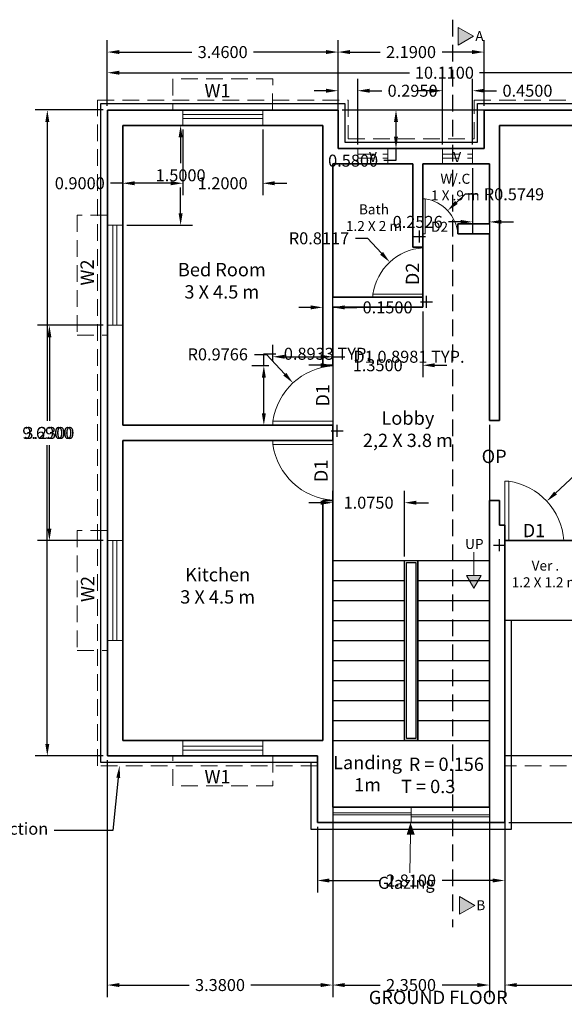
# Model space of a CAD drawing. Units: metres. Extents: x 5.2 to 41.7, y 12.2 to 37.4.
# Tile 3 of 6: x 19.4 to 27.6, y 12.2 to 27. Entities that reach past the tile are written whole.
import ezdxf
from ezdxf import colors
from ezdxf.entities.mleader import LeaderData, LeaderLine
from ezdxf.math import Vec2, Vec3

# ---------------------------------------------------------------- set-up
doc = ezdxf.new("R2010")
doc.units = ezdxf.units.M
doc.header["$MEASUREMENT"] = 0
doc.linetypes.add('HIDDEN', pattern=[0.375, 0.25, -0.125])
for name, color, linetype, lineweight in [('A-ANNO-DIMS', 2, 'Continuous', 18), ('A-ANNO-SYMB', 1, 'Continuous', 18), ('A-ANNO-SYMB-CUT', 3, 'HIDDEN', 25), ('A-ANNO-TEXT', 3, 'Continuous', 18), ('A-AREA-IDEN', 3, 'Continuous', 18), ('A-DOOR', 4, 'Continuous', 18), ('A-FLOR-PLIN', 7, 'Continuous', 25), ('A-FLOR-STRS', 7, 'Continuous', 25), ('A-ROOF-OVHD', 252, 'HIDDEN', 18), ('A-WALL', 7, 'Continuous', 35)]:
    doc.layers.add(name, color=color, linetype=linetype, lineweight=lineweight)
doc.layers.add('A-GLAZ', color=51, linetype='Continuous', lineweight=18, true_color=0xf7f281)
doc.layers.add('A-GLAZ-HIDN', color=51, linetype='HIDDEN', lineweight=18, true_color=0xf7f281)
doc.styles.get("Standard").update_dxf_attribs({"font": 'arial.ttf'})
doc.dimstyles.get("Standard").update_dxf_attribs({"dimtxt": 0.18, "dimasz": 0.18, "dimexe": 0.18, "dimexo": 0.0625, "dimgap": 0.09, "dimtad": 0, "dimtih": 1, "dimtoh": 1, "dimdec": 4, "dimzin": 0, "dimdsep": 46, "dimtxsty": 'Standard', "dimcen": 0.09, "dimadec": 0, "dimazin": 0, "dimtfac": 1, "dimtdec": 4, "dimtofl": 0, "dimtmove": 0, "dimatfit": 3, "dimfxl": 1, "dimtolj": 1, "dimtzin": 0, "dimarcsym": 0})

# ---------------------------------------------------------------- blocks, each defined once
blk = doc.blocks.new('*D2')
at = {"layer": 'A-ANNO-DIMS', "color": 0, "lineweight": -2, "transparency": 16777216}
for p, q in [((20.691, 25.661), (19.673, 25.661)), ((19.853, 25.481), (19.853, 20.998)), ((19.853, 16.151), (19.853, 20.634)), ((20.691, 15.971), (19.673, 15.971))]:
    blk.add_line(p, q, dxfattribs=at)
at = {"layer": 'A-ANNO-DIMS', "color": 0, "lineweight": 25, "transparency": 16777216}
for points in [[(19.823, 25.481), (19.883, 25.481), (19.853, 25.661)], [(19.823, 16.151), (19.883, 16.151), (19.853, 15.971)]]:
    blk.add_solid(points, dxfattribs=at)
at = {"layer": 'Defpoints', "color": 0, "lineweight": 25, "transparency": 16777216}
for p in [(19.853, 25.661), (20.753, 25.661), (20.753, 15.971)]:
    blk.add_point(p, dxfattribs=at)
at = {"layer": 'A-ANNO-DIMS', "color": 0, "transparency": 16777216, "insert": (19.853, 20.816), "char_height": 0.18, "attachment_point": 5}
blk.add_mtext('\\A1;9.6900', dxfattribs=at)
blk = doc.blocks.new('*D3')
at = {"layer": 'A-ANNO-DIMS', "color": 0, "lineweight": -2, "transparency": 16777216}
for p, q in [((20.753, 25.723), (20.753, 26.4)), ((30.863, 25.723), (30.863, 26.4)), ((20.933, 26.22), (25.283, 26.22)), ((30.683, 26.22), (26.333, 26.22))]:
    blk.add_line(p, q, dxfattribs=at)
at = {"layer": 'A-ANNO-DIMS', "color": 0, "lineweight": 25, "transparency": 16777216}
for points in [[(20.933, 26.25), (20.933, 26.19), (20.753, 26.22)], [(30.683, 26.25), (30.683, 26.19), (30.863, 26.22)]]:
    blk.add_solid(points, dxfattribs=at)
at = {"layer": 'Defpoints', "color": 0, "lineweight": 25, "transparency": 16777216}
for p in [(30.863, 26.22), (20.753, 25.661), (30.863, 25.661)]:
    blk.add_point(p, dxfattribs=at)
at = {"layer": 'A-ANNO-DIMS', "color": 0, "transparency": 16777216, "insert": (25.808, 26.22), "char_height": 0.18, "attachment_point": 5}
blk.add_mtext('\\A1;10.1100', dxfattribs=at)
blk = doc.blocks.new('WIN-W2-1500')
for p, q in [((0.23, 1.5), (0, 1.5)), ((0.085, 1.5), (0.085, 0)), ((0.145, 1.5), (0.145, 0)), ((0.23, 0), (0, 0))]:
    blk.add_line(p, q)
blk = doc.blocks.new('SUNSHADE-W2-1800')
blk.add_lwpolyline([(0.45, 1.65), (0.45, 1.8), (0, 1.8), (0, 0), (0.45, 0), (0.45, 0.15)])
blk = doc.blocks.new('DOOR-D1-900')
blk.add_lwpolyline([(0, 0), (0, 0.06), (0.898, 0.06), (0.898, 0)], close=True)
blk.add_arc((0.967, -0.081), 0.977, 94.015, 171.7193)
blk = doc.blocks.new('SECTION-DIRECTION')
h = blk.add_hatch(color=256)
h.dxf.hatch_style = 1
h.paths.add_polyline_path([(0, 0.266), (0, 0), (0.231, 0.133)])
blk.add_lwpolyline([(0.231, 0.133), (0, 0.266), (0, 0)], close=True)
blk = doc.blocks.new('STAIR-DIRECTION')
h = blk.add_hatch(color=256)
h.dxf.hatch_style = 1
h.paths.add_polyline_path([(0.219, 0.189), (0, 0.189), (0.044, 0.113), (0.175, 0.113)])
h.paths.add_polyline_path([(0.175, 0.113), (0.044, 0.113), (0.11, 0)])
blk.add_line((0.11, 0.189), (0.11, 0.542))
blk.add_lwpolyline([(0.11, 0), (0.219, 0.189), (0, 0.189)], close=True)
blk = doc.blocks.new('*D18')
at = {"layer": 'A-ANNO-DIMS', "color": 0, "lineweight": -2, "transparency": 16777216}
for p, q in [((23.235, 21.887), (23.235, 22.139)), ((24.133, 21.887), (24.133, 22.139)), ((23.415, 21.959), (23.953, 21.959)), ((24.133, 21.959), (24.313, 21.959))]:
    blk.add_line(p, q, dxfattribs=at)
at = {"layer": 'A-ANNO-DIMS', "color": 0, "lineweight": 25, "transparency": 16777216}
for points in [[(23.415, 21.989), (23.415, 21.929), (23.235, 21.959)], [(23.953, 21.989), (23.953, 21.929), (24.133, 21.959)]]:
    blk.add_solid(points, dxfattribs=at)
at = {"layer": 'Defpoints', "color": 0, "lineweight": 25, "transparency": 16777216}
for p in [(24.133, 21.959), (23.235, 21.824), (24.133, 21.824)]:
    blk.add_point(p, dxfattribs=at)
at = {"layer": 'A-ANNO-DIMS', "color": 0, "transparency": 16777216, "insert": (25.277, 21.959), "char_height": 0.18, "attachment_point": 5}
blk.add_mtext('\\A1;D1 0.8981 TYP.', dxfattribs=at)
blk = doc.blocks.new('*D19')
at = {"layer": 'A-ANNO-DIMS', "color": 0, "lineweight": -2, "transparency": 16777216}
for p, q in [((23.1, 21.824), (23.1, 22.004)), ((23.1, 22.004), (23.28, 22.004)), ((23.173, 21.824), (22.92, 21.824)), ((23.1, 21.111), (23.1, 21.644)), ((23.173, 20.931), (22.92, 20.931))]:
    blk.add_line(p, q, dxfattribs=at)
at = {"layer": 'A-ANNO-DIMS', "color": 0, "lineweight": 25, "transparency": 16777216}
for points in [[(23.07, 21.644), (23.13, 21.644), (23.1, 21.824)], [(23.07, 21.111), (23.13, 21.111), (23.1, 20.931)]]:
    blk.add_solid(points, dxfattribs=at)
at = {"layer": 'Defpoints', "color": 0, "lineweight": 25, "transparency": 16777216}
for p in [(23.1, 21.824), (23.235, 21.824), (23.235, 20.931)]:
    blk.add_point(p, dxfattribs=at)
at = {"layer": 'A-ANNO-DIMS', "color": 0, "transparency": 16777216, "insert": (24.053, 22.004), "char_height": 0.18, "attachment_point": 5}
blk.add_mtext('\\A1;0.8933 TYP.', dxfattribs=at)
blk = doc.blocks.new('*D26')
at = {"layer": 'A-ANNO-DIMS', "color": 0, "lineweight": -2, "transparency": 16777216}
for p, q in [((24.276, 25.661), (32.362, 25.661)), ((32.182, 25.481), (32.182, 20.498)), ((32.182, 15.151), (32.182, 20.134)), ((26.776, 14.971), (32.362, 14.971))]:
    blk.add_line(p, q, dxfattribs=at)
at = {"layer": 'A-ANNO-DIMS', "color": 0, "lineweight": 25, "transparency": 16777216}
for points in [[(32.152, 25.481), (32.212, 25.481), (32.182, 25.661)], [(32.152, 15.151), (32.212, 15.151), (32.182, 14.971)]]:
    blk.add_solid(points, dxfattribs=at)
at = {"layer": 'Defpoints', "color": 0, "lineweight": 25, "transparency": 16777216}
for p in [(24.213, 25.661), (26.713, 14.971), (32.182, 14.971)]:
    blk.add_point(p, dxfattribs=at)
at = {"layer": 'A-ANNO-DIMS', "color": 0, "transparency": 16777216, "insert": (32.182, 20.316), "char_height": 0.18, "attachment_point": 5}
blk.add_mtext('\\A1;10.6900', dxfattribs=at)
blk = doc.blocks.new('*D27')
at = {"layer": 'A-ANNO-DIMS', "color": 0, "lineweight": -2, "transparency": 16777216}
for p, q in [((23.903, 14.908), (23.903, 13.922)), ((26.713, 14.908), (26.713, 13.922)), ((24.083, 14.102), (24.843, 14.102)), ((26.533, 14.102), (25.773, 14.102))]:
    blk.add_line(p, q, dxfattribs=at)
at = {"layer": 'A-ANNO-DIMS', "color": 0, "lineweight": 25, "transparency": 16777216}
for points in [[(24.083, 14.132), (24.083, 14.072), (23.903, 14.102)], [(26.533, 14.132), (26.533, 14.072), (26.713, 14.102)]]:
    blk.add_solid(points, dxfattribs=at)
at = {"layer": 'Defpoints', "color": 0, "lineweight": 25, "transparency": 16777216}
for p in [(23.903, 14.971), (26.713, 14.971), (23.903, 14.102)]:
    blk.add_point(p, dxfattribs=at)
at = {"layer": 'A-ANNO-DIMS', "color": 0, "transparency": 16777216, "insert": (25.308, 14.102), "char_height": 0.18, "attachment_point": 5}
blk.add_mtext('\\A1;2.8100', dxfattribs=at)
blk = doc.blocks.new('*D28')
at = {"layer": 'A-ANNO-DIMS', "color": 0, "lineweight": -2, "transparency": 16777216}
for p, q in [((20.983, 25.368), (20.983, 24.382)), ((21.883, 25.368), (21.883, 24.382)), ((20.983, 24.562), (20.803, 24.562)), ((21.703, 24.562), (21.163, 24.562))]:
    blk.add_line(p, q, dxfattribs=at)
at = {"layer": 'A-ANNO-DIMS', "color": 0, "lineweight": 25, "transparency": 16777216}
for points in [[(21.163, 24.592), (21.163, 24.532), (20.983, 24.562)], [(21.703, 24.592), (21.703, 24.532), (21.883, 24.562)]]:
    blk.add_solid(points, dxfattribs=at)
at = {"layer": 'Defpoints', "color": 0, "lineweight": 25, "transparency": 16777216}
for p in [(20.983, 25.431), (21.883, 25.431), (20.983, 24.562)]:
    blk.add_point(p, dxfattribs=at)
at = {"layer": 'A-ANNO-DIMS', "color": 0, "transparency": 16777216, "insert": (20.34, 24.562), "char_height": 0.18, "attachment_point": 5}
blk.add_mtext('\\A1;0.9000', dxfattribs=at)
blk = doc.blocks.new('*D29')
at = {"layer": 'A-ANNO-DIMS', "color": 0, "lineweight": -2, "transparency": 16777216}
for p, q in [((21.883169, 25.368308), (21.883169, 24.381808)), ((23.083169, 25.368308), (23.083169, 24.381808)), ((21.703169, 24.561808), (21.523169, 24.561808)), ((23.263169, 24.561808), (23.443169, 24.561808))]:
    blk.add_line(p, q, dxfattribs=at)
at = {"layer": 'A-ANNO-DIMS', "color": 0, "lineweight": 25, "transparency": 16777216}
for points in [[(21.703169, 24.591808), (21.703169, 24.531808), (21.883169, 24.561808)], [(23.263169, 24.591808), (23.263169, 24.531808), (23.083169, 24.561808)]]:
    blk.add_solid(points, dxfattribs=at)
at = {"layer": 'Defpoints', "color": 0, "lineweight": 25, "transparency": 16777216}
for p in [(21.883169, 25.430808), (23.083169, 25.430808), (21.883169, 24.561808)]:
    blk.add_point(p, dxfattribs=at)
at = {"layer": 'A-ANNO-DIMS', "color": 0, "transparency": 16777216, "insert": (22.483169, 24.561808), "char_height": 0.18, "attachment_point": 5}
blk.add_mtext('\\A1;1.2000', dxfattribs=at)
blk = doc.blocks.new('*D30')
at = {"layer": 'A-ANNO-DIMS', "color": 0, "lineweight": -2, "transparency": 16777216}
for p, q in [((21.046, 25.431), (22.032, 25.431)), ((21.852, 25.251), (21.852, 24.863)), ((21.852, 24.111), (21.852, 24.499)), ((21.046, 23.931), (22.032, 23.931))]:
    blk.add_line(p, q, dxfattribs=at)
at = {"layer": 'A-ANNO-DIMS', "color": 0, "lineweight": 25, "transparency": 16777216}
for points in [[(21.822, 25.251), (21.882, 25.251), (21.852, 25.431)], [(21.822, 24.111), (21.882, 24.111), (21.852, 23.931)]]:
    blk.add_solid(points, dxfattribs=at)
at = {"layer": 'Defpoints', "color": 0, "lineweight": 25, "transparency": 16777216}
for p in [(20.983, 25.431), (20.983, 23.931), (21.852, 23.931)]:
    blk.add_point(p, dxfattribs=at)
at = {"layer": 'A-ANNO-DIMS', "color": 0, "transparency": 16777216, "insert": (21.852, 24.681), "char_height": 0.18, "attachment_point": 5}
blk.add_mtext('\\A1;1.5000', dxfattribs=at)
blk = doc.blocks.new('*D31')
at = {"layer": 'A-ANNO-DIMS', "color": 0, "lineweight": -2, "transparency": 16777216}
for p, q in [((20.691, 22.431), (19.704, 22.431)), ((19.884, 22.251), (19.884, 20.998)), ((19.884, 19.381), (19.884, 20.634)), ((20.691, 19.201), (19.704, 19.201))]:
    blk.add_line(p, q, dxfattribs=at)
at = {"layer": 'A-ANNO-DIMS', "color": 0, "lineweight": 25, "transparency": 16777216}
for points in [[(19.854, 22.251), (19.914, 22.251), (19.884, 22.431)], [(19.854, 19.381), (19.914, 19.381), (19.884, 19.201)]]:
    blk.add_solid(points, dxfattribs=at)
at = {"layer": 'Defpoints', "color": 0, "lineweight": 25, "transparency": 16777216}
for p in [(19.884, 22.431), (20.753, 22.431), (20.753, 19.201)]:
    blk.add_point(p, dxfattribs=at)
at = {"layer": 'A-ANNO-DIMS', "color": 0, "transparency": 16777216, "insert": (19.884, 20.816), "char_height": 0.18, "attachment_point": 5}
blk.add_mtext('\\A1;3.2300', dxfattribs=at)
blk = doc.blocks.new('*D34')
at = {"layer": 'A-ANNO-DIMS', "color": 0, "lineweight": -2, "transparency": 16777216}
for p, q in [((24.276, 25.661), (25.262, 25.661)), ((25.082, 25.481), (25.082, 25.261)), ((24.276, 25.081), (25.262, 25.081)), ((25.082, 25.081), (25.082, 24.901)), ((25.082, 24.901), (24.902, 24.901))]:
    blk.add_line(p, q, dxfattribs=at)
at = {"layer": 'A-ANNO-DIMS', "color": 0, "lineweight": 25, "transparency": 16777216}
for points in [[(25.052, 25.481), (25.112, 25.481), (25.082, 25.661)], [(25.052, 25.261), (25.112, 25.261), (25.082, 25.081)]]:
    blk.add_solid(points, dxfattribs=at)
at = {"layer": 'Defpoints', "color": 0, "lineweight": 25, "transparency": 16777216}
for p in [(24.213, 25.661), (24.213, 25.081), (25.082, 25.081)]:
    blk.add_point(p, dxfattribs=at)
at = {"layer": 'A-ANNO-DIMS', "color": 0, "transparency": 16777216, "insert": (24.439, 24.901), "char_height": 0.18, "attachment_point": 5}
blk.add_mtext('\\A1;0.5800', dxfattribs=at)
blk = doc.blocks.new('*D35')
at = {"layer": 'A-ANNO-DIMS', "color": 0, "lineweight": -2, "transparency": 16777216}
for p, q in [((25.781, 25.143), (25.781, 26.13)), ((26.231, 25.143), (26.231, 26.13)), ((25.601, 25.95), (25.421, 25.95)), ((26.411, 25.95), (26.591, 25.95))]:
    blk.add_line(p, q, dxfattribs=at)
at = {"layer": 'A-ANNO-DIMS', "color": 0, "lineweight": 25, "transparency": 16777216}
for points in [[(25.601, 25.98), (25.601, 25.92), (25.781, 25.95)], [(26.411, 25.98), (26.411, 25.92), (26.231, 25.95)]]:
    blk.add_solid(points, dxfattribs=at)
at = {"layer": 'Defpoints', "color": 0, "lineweight": 25, "transparency": 16777216}
for p in [(26.231, 25.95), (25.781, 25.081), (26.231, 25.081)]:
    blk.add_point(p, dxfattribs=at)
at = {"layer": 'A-ANNO-DIMS', "color": 0, "transparency": 16777216, "insert": (27.054, 25.95), "char_height": 0.18, "attachment_point": 5}
blk.add_mtext('\\A1;0.4500', dxfattribs=at)
blk = doc.blocks.new('*D36')
at = {"layer": 'A-ANNO-DIMS', "color": 0, "lineweight": -2, "transparency": 16777216}
for p, q in [((24.133169, 18.963308), (24.133169, 19.949808)), ((25.208169, 18.963308), (25.208169, 19.949808)), ((23.953169, 19.769808), (23.773169, 19.769808)), ((25.388169, 19.769808), (25.568169, 19.769808))]:
    blk.add_line(p, q, dxfattribs=at)
at = {"layer": 'A-ANNO-DIMS', "color": 0, "lineweight": 25, "transparency": 16777216}
for points in [[(23.953169, 19.799808), (23.953169, 19.739808), (24.133169, 19.769808)], [(25.388169, 19.799808), (25.388169, 19.739808), (25.208169, 19.769808)]]:
    blk.add_solid(points, dxfattribs=at)
at = {"layer": 'Defpoints', "color": 0, "lineweight": 25, "transparency": 16777216}
for p in [(25.208169, 19.769808), (24.133169, 18.900808), (25.208169, 18.900808)]:
    blk.add_point(p, dxfattribs=at)
at = {"layer": 'A-ANNO-DIMS', "color": 0, "transparency": 16777216, "insert": (24.670669, 19.769808), "char_height": 0.18, "attachment_point": 5}
blk.add_mtext('\\A1;1.0750', dxfattribs=at)
blk = doc.blocks.new('*D57')
at = {"layer": 'A-ANNO-DIMS', "color": 0, "lineweight": -2, "transparency": 16777216}
for p, q in [((20.753, 25.723), (20.753, 26.71)), ((24.213, 25.723), (24.213, 26.71)), ((20.933, 26.53), (22.02, 26.53)), ((24.033, 26.53), (22.946, 26.53))]:
    blk.add_line(p, q, dxfattribs=at)
at = {"layer": 'A-ANNO-DIMS', "color": 0, "lineweight": 25, "transparency": 16777216}
for points in [[(20.933, 26.56), (20.933, 26.5), (20.753, 26.53)], [(24.033, 26.56), (24.033, 26.5), (24.213, 26.53)]]:
    blk.add_solid(points, dxfattribs=at)
at = {"layer": 'Defpoints', "color": 0, "lineweight": 25, "transparency": 16777216}
for p in [(24.213, 26.53), (20.753, 25.661), (24.213, 25.661)]:
    blk.add_point(p, dxfattribs=at)
at = {"layer": 'A-ANNO-DIMS', "color": 0, "transparency": 16777216, "insert": (22.483, 26.53), "char_height": 0.18, "attachment_point": 5}
blk.add_mtext('\\A1;3.4600', dxfattribs=at)
blk = doc.blocks.new('*D58')
at = {"layer": 'A-ANNO-DIMS', "color": 0, "lineweight": -2, "transparency": 16777216}
for p, q in [((24.213, 25.723), (24.213, 26.71)), ((26.403, 25.723), (26.403, 26.71)), ((24.393, 26.53), (24.843, 26.53)), ((26.223, 26.53), (25.773, 26.53))]:
    blk.add_line(p, q, dxfattribs=at)
at = {"layer": 'A-ANNO-DIMS', "color": 0, "lineweight": 25, "transparency": 16777216}
for points in [[(24.393, 26.56), (24.393, 26.5), (24.213, 26.53)], [(26.223, 26.56), (26.223, 26.5), (26.403, 26.53)]]:
    blk.add_solid(points, dxfattribs=at)
at = {"layer": 'Defpoints', "color": 0, "lineweight": 25, "transparency": 16777216}
for p in [(26.403, 26.53), (24.213, 25.661), (26.403, 25.661)]:
    blk.add_point(p, dxfattribs=at)
at = {"layer": 'A-ANNO-DIMS', "color": 0, "transparency": 16777216, "insert": (25.308, 26.53), "char_height": 0.18, "attachment_point": 5}
blk.add_mtext('\\A1;2.1900', dxfattribs=at)
blk = doc.blocks.new('*D59')
at = {"layer": 'A-ANNO-DIMS', "color": 0, "lineweight": -2, "transparency": 16777216}
for p, q in [((20.753, 15.908), (20.753, 12.354)), ((24.133, 15.138), (24.133, 12.354)), ((20.933, 12.534), (21.98, 12.534)), ((23.953, 12.534), (22.906, 12.534))]:
    blk.add_line(p, q, dxfattribs=at)
at = {"layer": 'A-ANNO-DIMS', "color": 0, "lineweight": 25, "transparency": 16777216}
for points in [[(20.933, 12.564), (20.933, 12.504), (20.753, 12.534)], [(23.953, 12.564), (23.953, 12.504), (24.133, 12.534)]]:
    blk.add_solid(points, dxfattribs=at)
at = {"layer": 'Defpoints', "color": 0, "lineweight": 25, "transparency": 16777216}
for p in [(20.753, 15.971), (24.133, 15.201), (24.133, 12.534)]:
    blk.add_point(p, dxfattribs=at)
at = {"layer": 'A-ANNO-DIMS', "color": 0, "transparency": 16777216, "insert": (22.443, 12.534), "char_height": 0.18, "attachment_point": 5}
blk.add_mtext('\\A1;3.3800', dxfattribs=at)
blk = doc.blocks.new('*D60')
at = {"layer": 'A-ANNO-DIMS', "color": 0, "lineweight": -2, "transparency": 16777216}
for p, q in [((23.983, 21.893), (23.983, 22.88)), ((24.133, 21.893), (24.133, 22.88)), ((23.803, 22.7), (23.623, 22.7)), ((24.313, 22.7), (24.493, 22.7))]:
    blk.add_line(p, q, dxfattribs=at)
at = {"layer": 'A-ANNO-DIMS', "color": 0, "lineweight": 25, "transparency": 16777216}
for points in [[(23.803, 22.73), (23.803, 22.67), (23.983, 22.7)], [(24.313, 22.73), (24.313, 22.67), (24.133, 22.7)]]:
    blk.add_solid(points, dxfattribs=at)
at = {"layer": 'Defpoints', "color": 0, "lineweight": 25, "transparency": 16777216}
for p in [(24.133, 22.7), (23.983, 21.831), (24.133, 21.831)]:
    blk.add_point(p, dxfattribs=at)
at = {"layer": 'A-ANNO-DIMS', "color": 0, "transparency": 16777216, "insert": (24.956, 22.7), "char_height": 0.18, "attachment_point": 5}
blk.add_mtext('\\A1;0.1500', dxfattribs=at)
blk = doc.blocks.new('*D61')
at = {"layer": 'A-ANNO-DIMS', "color": 0, "lineweight": -2, "transparency": 16777216}
for p, q in [((24.133, 22.638), (24.133, 12.354)), ((26.483, 20.938), (26.483, 12.354)), ((24.313, 12.534), (24.843, 12.534)), ((26.303, 12.534), (25.773, 12.534))]:
    blk.add_line(p, q, dxfattribs=at)
at = {"layer": 'A-ANNO-DIMS', "color": 0, "lineweight": 25, "transparency": 16777216}
for points in [[(24.313, 12.564), (24.313, 12.504), (24.133, 12.534)], [(26.303, 12.564), (26.303, 12.504), (26.483, 12.534)]]:
    blk.add_solid(points, dxfattribs=at)
at = {"layer": 'Defpoints', "color": 0, "lineweight": 25, "transparency": 16777216}
for p in [(24.133, 22.701), (26.483, 21.001), (26.483, 12.534)]:
    blk.add_point(p, dxfattribs=at)
at = {"layer": 'A-ANNO-DIMS', "color": 0, "transparency": 16777216, "insert": (25.308, 12.534), "char_height": 0.18, "attachment_point": 5}
blk.add_mtext('\\A1;2.3500', dxfattribs=at)
blk = doc.blocks.new('*D62')
at = {"layer": 'A-ANNO-DIMS', "color": 0, "lineweight": -2, "transparency": 16777216}
for p, q in [((24.133169, 22.638308), (24.133169, 21.651808)), ((25.483169, 22.638308), (25.483169, 21.651808)), ((23.953169, 21.831808), (23.773169, 21.831808)), ((25.663169, 21.831808), (25.843169, 21.831808))]:
    blk.add_line(p, q, dxfattribs=at)
at = {"layer": 'A-ANNO-DIMS', "color": 0, "lineweight": 25, "transparency": 16777216}
for points in [[(23.953169, 21.861808), (23.953169, 21.801808), (24.133169, 21.831808)], [(25.663169, 21.861808), (25.663169, 21.801808), (25.483169, 21.831808)]]:
    blk.add_solid(points, dxfattribs=at)
at = {"layer": 'Defpoints', "color": 0, "lineweight": 25, "transparency": 16777216}
for p in [(24.133169, 22.700808), (25.483169, 22.700808), (24.133169, 21.831808)]:
    blk.add_point(p, dxfattribs=at)
at = {"layer": 'A-ANNO-DIMS', "color": 0, "transparency": 16777216, "insert": (24.808169, 21.831808), "char_height": 0.18, "attachment_point": 5}
blk.add_mtext('\\A1;1.3500', dxfattribs=at)
blk = doc.blocks.new('*D63')
at = {"layer": 'A-ANNO-DIMS', "color": 0, "lineweight": -2, "transparency": 16777216}
for p, q in [((24.213, 25.143), (24.213, 26.13)), ((24.508, 25.143), (24.508, 26.13)), ((24.033, 25.95), (23.853, 25.95)), ((24.688, 25.95), (24.868, 25.95))]:
    blk.add_line(p, q, dxfattribs=at)
at = {"layer": 'A-ANNO-DIMS', "color": 0, "lineweight": 25, "transparency": 16777216}
for points in [[(24.033, 25.98), (24.033, 25.92), (24.213, 25.95)], [(24.688, 25.98), (24.688, 25.92), (24.508, 25.95)]]:
    blk.add_solid(points, dxfattribs=at)
at = {"layer": 'Defpoints', "color": 0, "lineweight": 25, "transparency": 16777216}
for p in [(24.508, 25.95), (24.213, 25.081), (24.508, 25.081)]:
    blk.add_point(p, dxfattribs=at)
at = {"layer": 'A-ANNO-DIMS', "color": 0, "transparency": 16777216, "insert": (25.331, 25.95), "char_height": 0.18, "attachment_point": 5}
blk.add_mtext('\\A1;0.2950', dxfattribs=at)
blk = doc.blocks.new('*D64')
at = {"layer": 'A-ANNO-DIMS', "color": 0, "lineweight": -2, "transparency": 16777216}
for p, q in [((26.231, 24.788), (26.231, 23.802)), ((26.483, 24.788), (26.483, 23.802)), ((26.051, 23.982), (25.871, 23.982)), ((26.663, 23.982), (26.843, 23.982))]:
    blk.add_line(p, q, dxfattribs=at)
at = {"layer": 'A-ANNO-DIMS', "color": 0, "lineweight": 25, "transparency": 16777216}
for points in [[(26.051, 24.012), (26.051, 23.952), (26.231, 23.982)], [(26.663, 24.012), (26.663, 23.952), (26.483, 23.982)]]:
    blk.add_solid(points, dxfattribs=at)
at = {"layer": 'Defpoints', "color": 0, "lineweight": 25, "transparency": 16777216}
for p in [(26.231, 24.851), (26.483, 24.851), (26.231, 23.982)]:
    blk.add_point(p, dxfattribs=at)
at = {"layer": 'A-ANNO-DIMS', "color": 0, "transparency": 16777216, "insert": (25.407, 23.982), "char_height": 0.18, "attachment_point": 5}
blk.add_mtext('\\A1;0.2526', dxfattribs=at)
blk = doc.blocks.new('*D69')
at = {"layer": 'A-ANNO-DIMS', "color": 0, "lineweight": -2, "transparency": 16777216}
for p, q in [((30.461, 16.03), (30.461, 12.354)), ((26.713, 15.908), (26.713, 12.354)), ((26.893, 12.534), (28.124, 12.534)), ((30.281, 12.534), (29.05, 12.534))]:
    blk.add_line(p, q, dxfattribs=at)
at = {"layer": 'A-ANNO-DIMS', "color": 0, "lineweight": 25, "transparency": 16777216}
for points in [[(26.893, 12.564), (26.893, 12.504), (26.713, 12.534)], [(30.281, 12.564), (30.281, 12.504), (30.461, 12.534)]]:
    blk.add_solid(points, dxfattribs=at)
at = {"layer": 'Defpoints', "color": 0, "lineweight": 25, "transparency": 16777216}
for p in [(26.713, 15.971), (30.461, 16.092), (30.461, 12.534)]:
    blk.add_point(p, dxfattribs=at)
at = {"layer": 'A-ANNO-DIMS', "color": 0, "transparency": 16777216, "insert": (28.587, 12.534), "char_height": 0.18, "attachment_point": 5}
blk.add_mtext('\\A1;3.7480', dxfattribs=at)
blk = doc.blocks.new('*D92')
at = {"layer": 'A-ANNO-DIMS', "color": 0, "lineweight": -2, "transparency": 16777216}
for p, q in [((22.959, 21.995), (23.139, 21.995)), ((23.139, 21.995), (23.415, 21.698)), ((24.112, 20.85), (24.292, 20.85)), ((24.202, 20.76), (24.202, 20.94))]:
    blk.add_line(p, q, dxfattribs=at)
at = {"layer": 'A-ANNO-DIMS', "color": 0, "lineweight": 25, "transparency": 16777216}
blk.add_solid([(23.437, 21.718), (23.393, 21.677), (23.537, 21.566)], dxfattribs=at)
at = {"layer": 'Defpoints', "color": 0, "lineweight": 25, "transparency": 16777216}
for p in [(23.537, 21.566), (24.202, 20.85)]:
    blk.add_point(p, dxfattribs=at)
at = {"layer": 'A-ANNO-DIMS', "color": 0, "transparency": 16777216, "insert": (22.409, 21.995), "char_height": 0.18, "attachment_point": 5}
blk.add_mtext('\\A1;R0.9766', dxfattribs=at)
blk = doc.blocks.new('*D93')
at = {"layer": 'A-ANNO-DIMS', "color": 0, "lineweight": -2, "transparency": 16777216}
for p, q in [((27.769, 20.188), (27.475, 19.915)), ((27.949, 20.188), (27.769, 20.188)), ((26.633, 19.043), (26.633, 19.223)), ((26.543, 19.133), (26.723, 19.133))]:
    blk.add_line(p, q, dxfattribs=at)
at = {"layer": 'A-ANNO-DIMS', "color": 0, "lineweight": 25, "transparency": 16777216}
blk.add_solid([(27.455, 19.937), (27.496, 19.893), (27.343, 19.792)], dxfattribs=at)
at = {"layer": 'Defpoints', "color": 0, "lineweight": 25, "transparency": 16777216}
for p in [(27.343, 19.792), (26.633, 19.133)]:
    blk.add_point(p, dxfattribs=at)
at = {"layer": 'A-ANNO-DIMS', "color": 0, "transparency": 16777216, "insert": (28.482, 20.188), "char_height": 0.18, "attachment_point": 5}
blk.add_mtext('\\A1;R0.9691', dxfattribs=at)
blk = doc.blocks.new('*D94')
at = {"layer": 'A-ANNO-DIMS', "color": 0, "lineweight": -2, "transparency": 16777216}
for p, q in [((24.477, 23.736), (24.657, 23.736)), ((24.657, 23.736), (24.866, 23.511)), ((25.45, 22.784), (25.63, 22.784)), ((25.54, 22.694), (25.54, 22.874))]:
    blk.add_line(p, q, dxfattribs=at)
at = {"layer": 'A-ANNO-DIMS', "color": 0, "lineweight": 25, "transparency": 16777216}
blk.add_solid([(24.888, 23.531), (24.844, 23.49), (24.988, 23.379)], dxfattribs=at)
at = {"layer": 'Defpoints', "color": 0, "lineweight": 25, "transparency": 16777216}
for p in [(24.988, 23.379), (25.54, 22.784)]:
    blk.add_point(p, dxfattribs=at)
at = {"layer": 'A-ANNO-DIMS', "color": 0, "transparency": 16777216, "insert": (23.927, 23.736), "char_height": 0.18, "attachment_point": 5}
blk.add_mtext('\\A1;R0.8117', dxfattribs=at)
blk = doc.blocks.new('*D95')
at = {"layer": 'A-ANNO-DIMS', "color": 0, "lineweight": -2, "transparency": 16777216}
for p, q in [((26.121, 24.397), (25.989, 24.274)), ((26.301, 24.397), (26.121, 24.397)), ((25.436, 23.671), (25.436, 23.851)), ((25.346, 23.761), (25.526, 23.761))]:
    blk.add_line(p, q, dxfattribs=at)
at = {"layer": 'A-ANNO-DIMS', "color": 0, "lineweight": 25, "transparency": 16777216}
blk.add_solid([(25.968, 24.296), (26.009, 24.252), (25.857, 24.152)], dxfattribs=at)
at = {"layer": 'Defpoints', "color": 0, "lineweight": 25, "transparency": 16777216}
for p in [(25.857, 24.152), (25.436, 23.761)]:
    blk.add_point(p, dxfattribs=at)
at = {"layer": 'A-ANNO-DIMS', "color": 0, "transparency": 16777216, "insert": (26.851, 24.397), "char_height": 0.18, "attachment_point": 5}
blk.add_mtext('\\A1;R0.5749', dxfattribs=at)

msp = doc.modelspace()

# ---------------------------------------------------------------- linework, layer by layer
at = {"layer": 'A-ANNO-SYMB-CUT'}
msp.add_line((25.9275, 27.01562), (25.9275, 13.40349), dxfattribs=at)
at = {"layer": 'A-ANNO-TEXT'}
msp.add_lwpolyline([(25.30224, 14.79091), (25.29017, 14.21539)], dxfattribs=at)
msp.add_solid([(25.24336, 14.79205), (25.29882, 14.97081), (25.36418, 14.78992)], dxfattribs=at)
at = {"layer": 'A-DOOR'}
for points in [[(25.48317, 24.3295), (25.51835, 24.3295), (25.51835, 23.80081), (25.48317, 23.80081)], [(24.73673, 22.85081), (24.73673, 22.90049), (25.48317, 22.90049), (25.48317, 22.85081)], [(26.71317, 20.0919), (26.77247, 20.0919), (26.77247, 19.20081), (26.71317, 19.20081)]]:
    msp.add_lwpolyline(points, close=True, dxfattribs=at)
for centre, radius, start, end in [((25.43555, 23.76055), 0.57494, 4.015027, 81.719334), ((25.54, 22.78358), 0.81174, 94.015027, 171.719334), ((26.63291, 19.13296), 0.96905, 4.015027, 81.719334)]:
    msp.add_arc(centre, radius, start, end, dxfattribs=at)
at = {"layer": 'A-FLOR-PLIN'}
msp.add_line((30.86317, 15.97081), (26.71317, 15.97081), dxfattribs=at)
for points in [[(23.90317, 15.87081), (20.65317, 15.87081), (20.65317, 25.76081), (24.31317, 25.76081), (24.31317, 25.18081), (26.30317, 25.18081), (26.30317, 25.76081), (30.96317, 25.76081), (30.96317, 19.10081), (28.81317, 19.10081)], [(23.80317, 15.87081), (23.80317, 14.87081), (26.81317, 14.87081), (26.81317, 18.00081)]]:
    msp.add_lwpolyline(points, dxfattribs=at)
at = {"layer": 'A-FLOR-STRS'}
for p, q in [((24.13317, 18.90081), (25.20817, 18.90081)), ((25.20817, 16.20081), (25.20817, 18.90081)), ((25.40817, 16.20081), (25.40817, 18.90081)), ((25.40817, 18.90081), (26.48317, 18.90081)), ((24.13317, 18.60081), (25.20817, 18.60081)), ((25.40817, 18.60081), (26.48317, 18.60081)), ((24.13317, 18.30081), (25.20817, 18.30081)), ((25.40817, 18.30081), (26.48317, 18.30081)), ((24.13317, 18.00081), (25.20817, 18.00081)), ((25.40817, 18.00081), (26.48317, 18.00081)), ((28.81317, 18.00081), (26.71317, 18.00081)), ((24.13317, 17.70081), (25.20817, 17.70081)), ((25.40817, 17.70081), (26.48317, 17.70081)), ((24.13317, 17.40081), (25.20817, 17.40081)), ((25.40817, 17.40081), (26.48317, 17.40081)), ((24.13317, 17.10081), (25.20817, 17.10081)), ((25.40817, 17.10081), (26.48317, 17.10081)), ((24.13317, 16.80081), (25.20817, 16.80081)), ((25.40817, 16.80081), (26.48317, 16.80081)), ((24.13317, 16.50081), (25.20817, 16.50081)), ((25.40817, 16.50081), (26.48317, 16.50081)), ((24.13317, 16.20081), (26.48317, 16.20081))]:
    msp.add_line(p, q, dxfattribs=at)
for points in [[(25.20817, 18.90106), (25.40817, 18.90106), (25.40817, 16.20081), (25.20817, 16.20081)], [(25.23817, 18.87128), (25.37817, 18.87128), (25.37817, 16.23081), (25.23817, 16.23081)]]:
    msp.add_lwpolyline(points, close=True, dxfattribs=at)
at = {"layer": 'A-GLAZ'}
for p, q in [((21.88317, 25.43081), (21.88317, 25.66081)), ((21.88317, 25.5936), (23.08317, 25.5936)), ((23.08317, 25.43081), (23.08317, 25.66081)), ((21.88317, 25.5336), (23.08317, 25.5336)), ((24.50817, 24.85081), (24.50817, 25.08081)), ((24.95817, 24.85081), (24.95817, 25.08081)), ((25.78061, 24.85081), (25.78061, 25.08081)), ((26.23061, 24.85081), (26.23061, 25.08081)), ((21.88317, 16.20081), (21.88317, 15.97081)), ((21.88317, 16.11581), (23.08317, 16.11581)), ((23.08317, 16.20081), (23.08317, 15.97081)), ((21.88317, 16.05581), (23.08317, 16.05581)), ((24.13317, 15.20081), (24.13317, 14.97081)), ((24.13317, 15.11581), (25.30817, 15.11581)), ((24.13317, 15.08581), (26.48317, 15.08581)), ((25.30817, 15.20081), (25.30817, 14.97081)), ((26.48317, 15.20081), (26.48317, 14.97081)), ((25.30817, 15.05581), (26.48317, 15.05581))]:
    msp.add_line(p, q, dxfattribs=at)
at = {"layer": 'A-GLAZ-HIDN'}
for p, q in [((24.50817, 24.99581), (24.95817, 24.99581)), ((25.78061, 24.99581), (26.23061, 24.99581)), ((24.50817, 24.93581), (24.95817, 24.93581)), ((25.78061, 24.93581), (26.23061, 24.93581))]:
    msp.add_line(p, q, dxfattribs=at)
at = {"layer": 'A-ROOF-OVHD'}
for points in [[(23.08317, 25.66081), (23.23165, 25.66081), (23.23317, 26.1286), (21.73317, 26.1286), (21.73303, 25.66081), (21.88317, 25.66081)], [(23.90317, 15.82081), (20.60317, 15.82081), (20.60317, 25.81081), (24.36317, 25.81081), (24.36317, 25.23081), (26.25317, 25.23081), (26.25317, 25.81081), (31.01317, 25.81081), (31.01317, 15.82081), (26.71317, 15.82081)], [(23.08317, 15.97081), (23.23317, 15.97081), (23.23317, 15.52081), (21.73317, 15.52081), (21.73317, 15.97081), (21.88317, 15.97081)]]:
    msp.add_lwpolyline(points, dxfattribs=at)
at = {"layer": 'A-WALL'}
for p, q in [((20.75317, 25.66081), (20.75317, 15.97081)), ((24.21317, 25.66081), (20.75317, 25.66081)), ((24.21317, 25.08081), (24.21317, 25.66081)), ((30.86317, 25.66081), (26.40317, 25.66081)), ((26.40317, 25.08081), (26.40317, 25.66081)), ((20.98317, 25.43081), (20.98317, 20.93081)), ((23.98317, 25.43081), (20.98317, 25.43081)), ((23.98317, 21.83081), (23.98317, 25.43081)), ((30.63317, 25.43081), (26.63317, 25.43081)), ((26.63317, 21.00081), (26.63317, 25.43081)), ((24.21317, 25.08081), (26.40317, 25.08081)), ((24.13317, 24.85081), (25.33317, 24.85081)), ((24.13317, 22.85081), (24.13317, 24.85081)), ((25.33317, 23.60081), (25.33317, 24.85081)), ((25.48317, 22.70081), (25.48317, 24.85081)), ((25.48317, 24.85081), (26.48317, 24.85081)), ((26.48317, 23.95081), (26.48317, 24.85081)), ((26.00908, 23.80081), (26.00884, 23.95081)), ((26.00884, 23.95081), (26.48317, 23.95081)), ((26.00908, 23.80164), (26.48317, 23.80081)), ((26.48317, 21.00081), (26.48317, 23.80081)), ((25.33317, 23.60081), (25.48317, 23.60081)), ((24.13317, 22.85081), (25.48317, 22.85081)), ((24.13317, 22.70081), (25.48317, 22.70081)), ((24.13317, 21.83081), (24.13317, 22.70081)), ((24.13317, 21.83081), (23.98317, 21.83081)), ((26.48317, 21.00081), (26.63317, 21.00081)), ((24.13317, 20.93081), (20.98317, 20.93081)), ((24.13317, 20.70081), (24.13317, 20.93081)), ((24.13317, 20.70081), (20.98317, 20.70081)), ((20.98317, 20.70081), (20.98317, 16.20081)), ((23.98317, 16.20081), (23.98317, 19.80081)), ((24.13317, 19.80081), (23.98317, 19.80081)), ((24.13317, 15.20081), (24.13317, 19.80081)), ((26.48317, 15.20081), (26.48317, 19.80081)), ((26.48317, 19.80081), (26.63317, 19.80081)), ((26.63317, 19.43081), (26.63317, 19.80081)), ((26.71317, 19.43081), (26.63317, 19.43081)), ((26.71317, 14.97081), (26.71317, 19.43081)), ((30.86317, 19.20081), (26.71317, 19.20081)), ((20.98317, 16.20081), (23.98317, 16.20081)), ((20.75317, 15.97081), (23.90317, 15.97081)), ((23.90317, 14.97081), (23.90317, 15.97081)), ((24.13317, 15.20081), (26.48317, 15.20081)), ((23.90317, 14.97081), (26.71317, 14.97081))]:
    msp.add_line(p, q, dxfattribs=at)

# ---------------------------------------------------------------- block references
at = {"layer": 'A-ANNO-SYMB'}
for name, p in [('SECTION-DIRECTION', (26.015, 26.633)), ('STAIR-DIRECTION', (26.141, 18.488)), ('SECTION-DIRECTION', (26.03492, 13.59548))]:
    msp.add_blockref(name, p, dxfattribs=at)
at = {"layer": 'A-DOOR'}
msp.add_blockref('DOOR-D1-900', (23.235, 20.931), dxfattribs=at)
at = {"layer": 'A-DOOR', "extrusion": (0, 0, -1), "zscale": -1, "rotation": 180}
msp.add_blockref('DOOR-D1-900', (-23.235, 20.70062), dxfattribs=at)
at = {"layer": 'A-GLAZ'}
for p in [(20.753, 22.431), (20.753, 17.701)]:
    msp.add_blockref('WIN-W2-1500', p, dxfattribs=at)
at = {"layer": 'A-ROOF-OVHD'}
for p in [(20.303, 22.281), (20.303, 17.551)]:
    msp.add_blockref('SUNSHADE-W2-1800', p, dxfattribs=at)

# ---------------------------------------------------------------- texts
at = {"layer": 'A-ANNO-TEXT', "attachment_point": 1}
for s, width, insert, char_height in [('\\pxqc;{A}', 1.8483261, (25.40982, 26.84414), 0.15), ('\\pxqc;{W1 }', 1.8483261, (21.48154, 26.05023), 0.2), ('\\pxqc;{V}', 1.8483261, (23.81233, 25.0329), 0.15), ('\\pxqc;{V}', 1.8483261, (25.07508, 25.02857), 0.15), ('\\pxqc;{D2}', 1.8483261, (24.81197, 23.98325), 0.15), ('\\pxqc;{OP}', 1.8483261, (25.63019, 20.56488), 0.2), ('\\pxqc;{D1 }', 1.8483261, (26.22747, 19.45253), 0.2), ('\\pxqc;{UP }', 1.8483261, (25.33299, 19.22594), 0.15), ('\\pxqc;{R = 0.156 \\P\\pq*;    T = 0.3 }', 1.8483261, (24.91263, 15.94585), 0.2), ('\\pxqc;{W1 }', 1.8483261, (21.48154, 15.76023), 0.2), ('\\pxqc;{B}', 1.8483261, (25.42974, 13.80662), 0.15), ('\\pxqc;{GROUND FLOOR }', 2.8220899, (24.30501, 12.44843), 0.2)]:
    msp.add_mtext_dynamic_manual_height_columns(s, width=width, gutter_width=1, heights=[0], dxfattribs=dict(at, insert=insert, char_height=char_height))
at = {"layer": 'A-ANNO-TEXT', "char_height": 0.2, "attachment_point": 1, "rotation": 90}
for s, insert in [('\\pxqc;{W2 }', (20.35072, 22.29879)), ('\\pxqc;{D2}', (25.22968, 22.27775)), ('\\pxqc;{D1 }', (23.88329, 20.45687)), ('\\pxqc;{D1 }', (23.85801, 19.32238)), ('\\pxqc;{W2 }', (20.35721, 17.55081))]:
    msp.add_mtext_dynamic_manual_height_columns(s, width=1.8483261, gutter_width=1, heights=[0], dxfattribs=dict(at, insert=insert))
at = {"layer": 'A-ANNO-TEXT', "insert": (25.66202, 14.15727), "char_height": 0.18, "attachment_point": 3}
msp.add_mtext('Glazing  ', dxfattribs=at)
at = {"layer": 'A-AREA-IDEN', "attachment_point": 1}
for s, insert, char_height in [('\\pxqc;{W/.C \\P1 X .9 m}', (25.04801, 24.70425), 0.15), ('\\pxqc;{Bath \\P1.2 X 2 m}', (23.82747, 24.24572), 0.15), ('\\pxqc;{Bed Room \\P3 X 4.5 m }', (21.54593, 23.36586), 0.2), ('\\pxqc;{Lobby \\P2,2 X 3.8 m}', (24.3362, 21.13859), 0.2), ('\\pxqc;{Kitchen  \\P3 X 4.5 m }', (21.48366, 18.7898), 0.2), ('\\pxqc;{Ver .\\P1.2 X 1.2 m}', (26.39866, 18.90081), 0.15), ('\\pxqc;{Landing  \\P1m }', (23.7313, 15.97081), 0.2)]:
    msp.add_mtext_dynamic_manual_height_columns(s, width=1.8483261, gutter_width=1, heights=[0], dxfattribs=dict(at, insert=insert, char_height=char_height))

# ---------------------------------------------------------------- dimensions: what is measured, and where the dimension line sits
at = {"layer": 'A-ANNO-DIMS'}
for base, p1, p2, override, picture, middle in [((24.21317, 26.52981), (20.75317, 25.66081), (24.21317, 25.66081), {"dimdec": 4, "dimlfac": 1, "dimrnd": 0, "dimzin": 0, "dimdsep": 46, "dimlunit": 2}, '*D57', (22.48317, 26.52981)), ((26.40317, 26.52981), (24.21317, 25.66081), (26.40317, 25.66081), {"dimdec": 4, "dimlfac": 1, "dimrnd": 0, "dimzin": 0, "dimdsep": 46, "dimlunit": 2}, '*D58', (25.30817, 26.52981)), ((30.86317, 26.22005), (20.75317, 25.66081), (30.86317, 25.66081), {"dimclrd": 0, "dimclre": 0, "dimclrt": 0}, '*D3', (25.80817, 26.22005)), ((24.50817, 25.94981), (24.21317, 25.08081), (24.50817, 25.08081), {"dimdec": 4, "dimlfac": 1, "dimrnd": 0, "dimzin": 0, "dimdsep": 46, "dimlunit": 2}, '*D63', (25.33149, 25.94981)), ((26.23061, 25.94981), (25.78061, 25.08081), (26.23061, 25.08081), {"dimdec": 4, "dimlfac": 1, "dimrnd": 0, "dimzin": 0, "dimdsep": 46, "dimlunit": 2}, '*D35', (27.05393, 25.94981)), ((24.13317, 22.69981), (23.98317, 21.83081), (24.13317, 21.83081), {"dimdec": 4, "dimlfac": 1, "dimrnd": 0, "dimzin": 0, "dimdsep": 46, "dimlunit": 2}, '*D60', (24.95649, 22.69981)), ((26.48317, 12.53449), (24.13317, 22.70081), (26.48317, 21.00081), {"dimdec": 4, "dimlfac": 1, "dimrnd": 0, "dimzin": 0, "dimdsep": 46, "dimlunit": 2}, '*D61', (25.30817, 12.53449)), ((25.20817, 19.76981), (24.13317, 18.90081), (25.20817, 18.90081), {"dimdec": 4, "dimlfac": 1, "dimrnd": 0, "dimzin": 0, "dimdsep": 46, "dimlunit": 2}, '*D36', (24.67067, 19.76981)), ((24.13317, 12.53449), (20.75317, 15.97081), (24.13317, 15.20081), {"dimdec": 4, "dimlfac": 1, "dimrnd": 0, "dimzin": 0, "dimdsep": 46, "dimlunit": 2}, '*D59', (22.44317, 12.53449)), ((30.46113, 12.53449), (26.71317, 15.97081), (30.46113, 16.09214), {"dimdec": 4, "dimlfac": 1, "dimrnd": 0, "dimzin": 0, "dimdsep": 46, "dimlunit": 2}, '*D69', (28.58715, 12.53449))]:
    dim = msp.add_linear_dim(base=base, p1=p1, p2=p2, dimstyle='Standard', override=override, dxfattribs=at)
    dim.commit()
    dim.dimension.update_dxf_attribs({"geometry": picture, "text_midpoint": middle})
for base, p1, p2, angle, override, picture, middle in [((19.8529, 25.66081), (20.75317, 15.97081), (20.75317, 25.66081), 90, {"dimclrd": 0, "dimclre": 0, "dimclrt": 0}, '*D2', (19.8529, 20.81581)), ((25.08217, 25.08081), (24.21317, 25.66081), (24.21317, 25.08081), 270, {"dimdec": 4, "dimlfac": 1, "dimrnd": 0, "dimzin": 0, "dimdsep": 46, "dimlunit": 2}, '*D34', (24.43885, 24.90081)), ((32.18217, 14.97081), (24.21317, 25.66081), (26.71317, 14.97081), 90, {"dimdec": 4, "dimlfac": 1, "dimrnd": 0, "dimzin": 0, "dimdsep": 46, "dimlunit": 2}, '*D26', (32.18217, 20.31581)), ((20.98317, 24.56181), (21.88317, 25.43081), (20.98317, 25.43081), 180, {"dimdec": 4, "dimlfac": 1, "dimrnd": 0, "dimzin": 0, "dimdsep": 46, "dimlunit": 2}, '*D28', (20.33985, 24.56181)), ((21.85217, 23.93081), (20.98317, 25.43081), (20.98317, 23.93081), 270, {"dimdec": 4, "dimlfac": 1, "dimrnd": 0, "dimzin": 0, "dimdsep": 46, "dimlunit": 2}, '*D30', (21.85217, 24.68081)), ((21.88317, 24.56181), (23.08317, 25.43081), (21.88317, 25.43081), 180, {"dimdec": 4, "dimlfac": 1, "dimrnd": 0, "dimzin": 0, "dimdsep": 46, "dimlunit": 2}, '*D29', (22.48317, 24.56181)), ((26.23061, 23.98181), (26.48317, 24.85081), (26.23061, 24.85081), 180, {"dimdec": 4, "dimlfac": 1, "dimrnd": 0, "dimzin": 0, "dimdsep": 46, "dimlunit": 2}, '*D64', (25.40704, 23.98181)), ((24.13317, 21.83181), (25.48317, 22.70081), (24.13317, 22.70081), 180, {"dimdec": 4, "dimlfac": 1, "dimrnd": 0, "dimzin": 0, "dimdsep": 46, "dimlunit": 2}, '*D62', (24.80817, 21.83181)), ((19.88417, 22.43081), (20.75317, 19.20081), (20.75317, 22.43081), 90, {"dimdec": 4, "dimlfac": 1, "dimrnd": 0, "dimzin": 0, "dimdsep": 46, "dimlunit": 2}, '*D31', (19.88417, 20.81581)), ((23.90317, 14.10181), (26.71317, 14.97081), (23.90317, 14.97081), 180, {"dimdec": 4, "dimlfac": 1, "dimrnd": 0, "dimzin": 0, "dimdsep": 46, "dimlunit": 2}, '*D27', (25.30817, 14.10181))]:
    dim = msp.add_linear_dim(base=base, p1=p1, p2=p2, angle=angle, dimstyle='Standard', override=override, dxfattribs=at)
    dim.commit()
    dim.dimension.update_dxf_attribs({"geometry": picture, "text_midpoint": middle})
dim = msp.add_radius_dim(center=(25.43555, 23.76055), mpoint=(25.85681, 24.15183), dimstyle='Standard', override={"dimdec": 4, "dimlfac": 1, "dimrnd": 0, "dimzin": 0, "dimdsep": 46, "dimlunit": 2}, dxfattribs=at)
dim.commit()
dim.dimension.update_dxf_attribs({"geometry": '*D95', "text_midpoint": (26.85053, 24.39682)})
for center, mpoint, picture, middle in [((25.54, 22.78358), (24.98813, 23.37886), '*D94', (23.92725, 23.73602)), ((24.20155, 20.84992), (23.53721, 21.56577), '*D92', (22.40891, 21.99528)), ((26.632909, 19.132957), (27.343186, 19.792173), '*D93', (28.481739, 20.187702))]:
    dim = msp.add_radius_dim(center=center, mpoint=mpoint, dimstyle='Standard', override={"dimdec": 4, "dimlfac": 1, "dimrnd": 0, "dimzin": 0, "dimdsep": 46, "dimlunit": 2}, dxfattribs=at)
    dim.commit()
    dim.dimension.update_dxf_attribs({"geometry": picture, "text_midpoint": middle, "dimtype": 164})
dim = msp.add_linear_dim(base=(24.13317, 21.95885), p1=(23.23511, 21.82415), p2=(24.13317, 21.82415), text='D1 <> TYP.', dimstyle='Standard', override={"dimdec": 4, "dimlfac": 1, "dimrnd": 0, "dimzin": 0, "dimdsep": 46, "dimlunit": 2}, dxfattribs=at)
dim.commit()
dim.dimension.update_dxf_attribs({"geometry": '*D18', "text_midpoint": (25.27714, 21.95885)})
dim = msp.add_linear_dim(base=(23.1004, 21.82415), p1=(23.23511, 20.93081), p2=(23.23511, 21.82415), angle=90, text='<> TYP.', dimstyle='Standard', override={"dimdec": 4, "dimlfac": 1, "dimrnd": 0, "dimzin": 0, "dimdsep": 46, "dimlunit": 2}, dxfattribs=at)
dim.commit()
dim.dimension.update_dxf_attribs({"geometry": '*D19', "text_midpoint": (24.0532, 22.00415)})

# ---------------------------------------------------------------- leaders
at = {"layer": 'A-ANNO-TEXT'}
ml = msp.add_multileader_mtext('Standard', dxfattribs=at)
ml.set_content('Slab  projection ', color=256)
ml.set_leader_properties()
ml.build(insert=Vec2(0, 0))
ml.multileader.update_dxf_attribs({"dogleg_length": 0.36, "arrow_head_size": 0.18})
ctx = ml.context
ctx.base_point, ctx.char_height, ctx.arrow_head_size, ctx.landing_gap_size, ctx.plane_origin = Vec3(18.07181, 14.85251), 0.18, 0.18, 0.09, Vec3(20.72542, 15.63365)
ctx.text_align_type = 2
notes = []
notes.append((ctx, [(1, (1, 1, 0), (20.8335, 14.85251), (-1, 0), 0.87697, [(0, [(20.93558, 15.82081)], 0, [])])]))
ctx.mtext.insert, ctx.mtext.alignment, ctx.mtext.flow_direction = Vec3(19.86653, 14.96897), 3, 5
for ctx, leaders in notes:
    for number, flags, end, landing, length, lines in leaders:
        leader = LeaderData()
        leader.index, (leader.has_last_leader_line, leader.has_dogleg_vector, leader.attachment_direction) = number, flags
        leader.last_leader_point, leader.dogleg_vector, leader.dogleg_length = Vec3(end), Vec3(landing), length
        for number, points, colour, breaks in lines:
            line = LeaderLine()
            line.index, line.vertices, line.color, line.breaks = number, Vec3.list(points), colors.encode_raw_color(colour), breaks
            leader.lines.append(line)
        ctx.leaders.append(leader)

doc.saveas('drawing.dxf')
